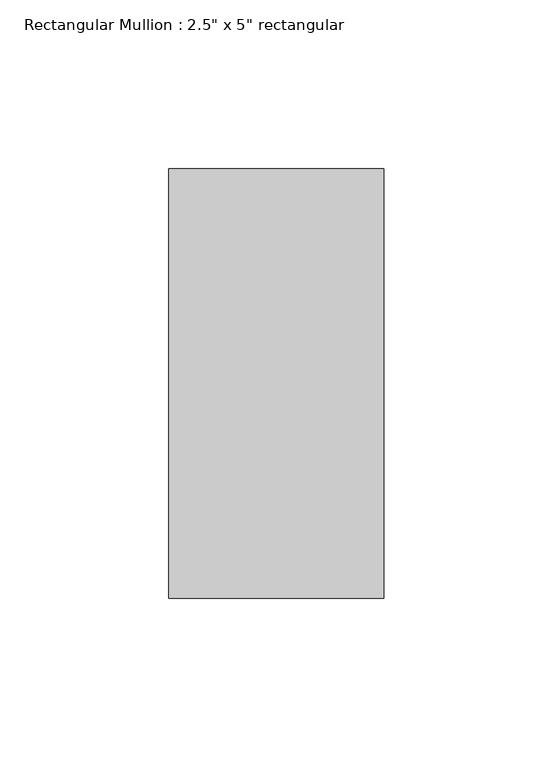
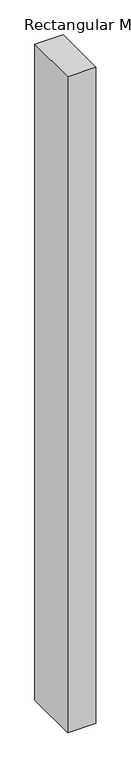
"""IFC4 building model written with IfcOpenShell, lengths in millimetres: member geometry."""

from ifc_helpers import new_model, si_unit, frame, origin, place, context, project, spatial, polyline, outline, extrude, source, transform, mapped, element, save


def member_e7529cf5(model_context):
    return source(origin(), model_context, "Body", "SweptSolid", [
        extrude(outline(polyline([(31.75, 63.5), (31.75, -63.5), (-31.75, -63.5), (-31.75, 63.5), (31.75, 63.5)])), frame((0.0, 0.0, -1557.357611), z_axis=(0.0, 0.0, 1.0), x_axis=(1.0, 0.0, 0.0)), (0.0, 0.0, 1.0), 1557.357611),
    ])


if __name__ == "__main__":
    model = new_model("IFC4")
    model_context = context("Model", 3, world=origin())
    ifc_project = project(units=[si_unit("LENGTHUNIT", "METRE", prefix="MILLI")], contexts=[model_context])
    site = spatial("IfcSite", under=ifc_project)
    building = spatial("IfcBuilding", under=site)
    placement = place(None, origin())
    member_shape = member_e7529cf5(model_context)
    element("IfcMember", 1, ObjectType="Rectangular Mullion : 2.5\" x 5\" rectangular", at=placement, inside=building, context=model_context, shape_type="MappedRepresentation", body=[
        mapped(member_shape, transform((0.0, 0.0, 0.0), x_axis=(1.0, 0.0, 0.0), y_axis=(0.0, 1.0, 0.0), z_axis=(0.0, 0.0, 1.0))),
    ])
    save(model, "model.ifc")

# Revit data of these elements
# Type "Rectangular Mullion : 2.5\" x 5\" rectangular"
#   built-in parameter 1007304 = 0.416667 (stored number, unit not read)
#   built-in parameter 1007301 = 0.104167 (stored number, unit not read)
#   built-in parameter 1007300 = 0.104167 (stored number, unit not read)
# Element 1 (IfcMember, "Rectangular Mullion : 2.5\" x 5\" rectangular")
#   Materials on its faces: "Aluminum"
# Materials
#   "Aluminum": class "Metal", colour RGB 247 247 247, transparency 0, Description = "Aluminum 6061", Cost = 0
